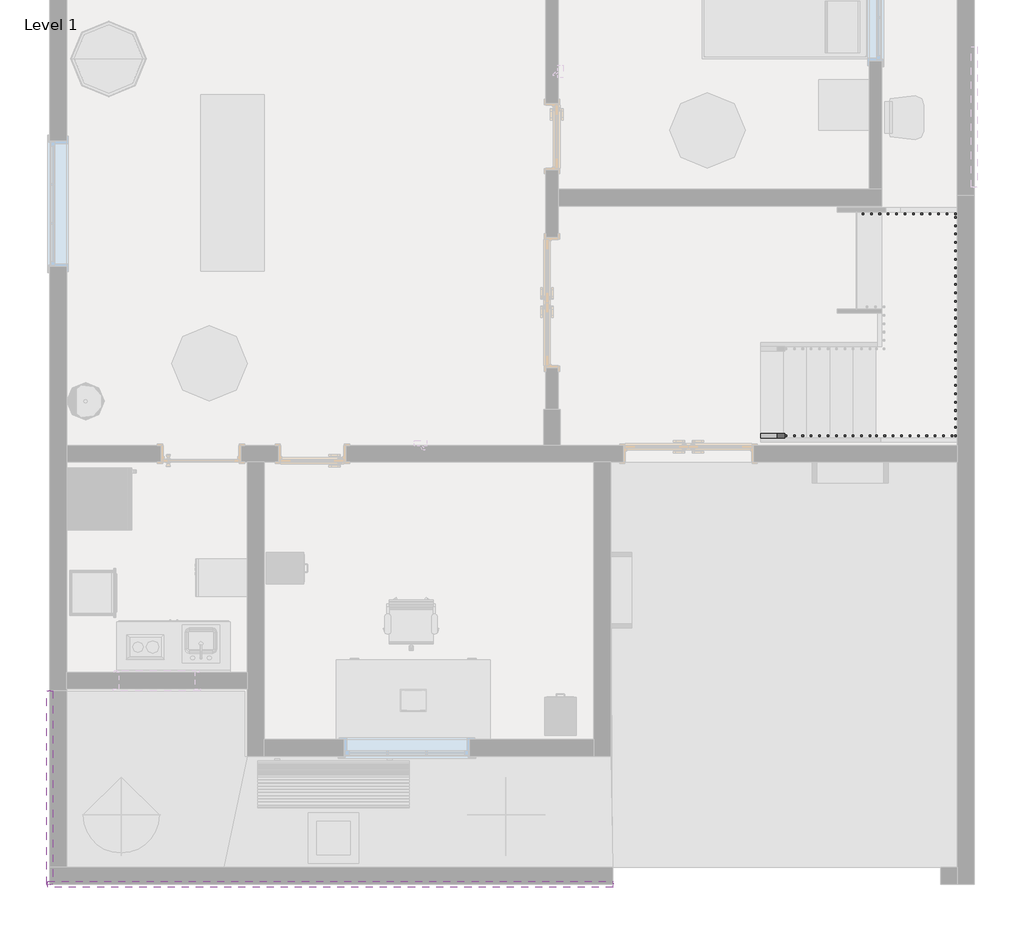
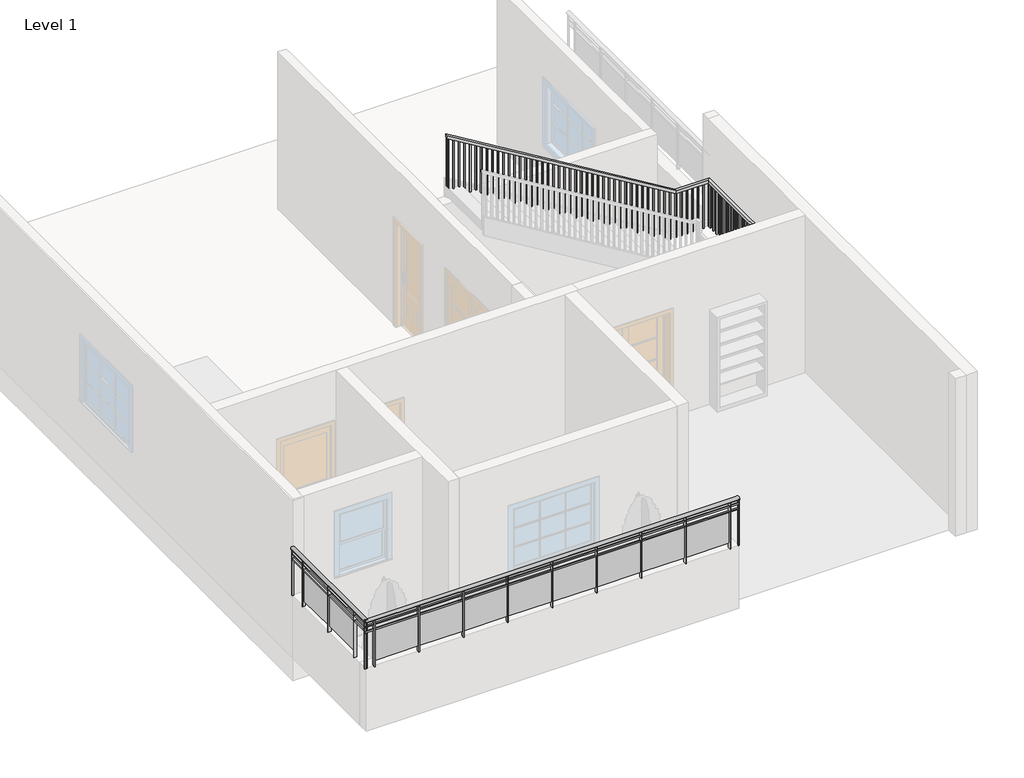
# One storey, part 2 of 4: 3 railings.
"""IFC4 building model written with IfcOpenShell, lengths in millimetres."""

from ifc_helpers import new_model, si_unit, point, frame, origin, place, context, project, spatial, polyline, ellipse_curve, trimmed, outline, extrude, faceted_brep, element, save
from ifc_brep_helpers import plane_surface, extruded_surface, advanced_brep

model = new_model("IFC4")

# Units and contexts
model_context = context("Model", 3, world=origin())
ifc_project = project(units=[si_unit("LENGTHUNIT", "METRE", prefix="MILLI")], contexts=[model_context])

# Site, building, storey
site = spatial("IfcSite", under=ifc_project)
building = spatial("IfcBuilding", under=site)
storey = spatial("IfcBuildingStorey", under=building, Name="Level 1", Elevation=0.0)

# Railings
placement = place(None, origin())
element("IfcRailing", 1, ObjectType="Glass Panel - Bottom Fill", at=placement, inside=storey, context=model_context, shape_type="SolidModel", body=[
    advanced_brep(
    [(-11727.0886283, -588.2425054, 2133.6), (-11803.2886283, -588.2425054, 2133.6), (-11727.0886283, -2925.0425054, 2133.6), (-11803.2886283, -2925.0425054, 2133.6)],
    [
        (0, 1, ellipse_curve(frame((-11765.1886283, -588.2425054, 2133.6), z_axis=(0.0, 1.0, 0.0), x_axis=(-1.0, 0.0, 0.0)), 38.1, 28.575)),
        (1, 0, ellipse_curve(frame((-11765.1886283, -588.2425054, 2133.6), z_axis=(0.0, 1.0, 0.0), x_axis=(-1.0, 0.0, 0.0)), 38.1, 28.575)),
        (2, 3, ellipse_curve(frame((-11765.1886283, -2925.0425054, 2133.6), z_axis=(0.0, -1.0, 0.0), x_axis=(-1.0, 0.0, 0.0)), 38.1, 28.575)),
        (3, 2, ellipse_curve(frame((-11765.1886283, -2925.0425054, 2133.6), z_axis=(0.0, -1.0, 0.0), x_axis=(-1.0, 0.0, 0.0)), 38.1, 28.575)),
        (0, 2),
        (3, 1),
    ],
    [
        plane_surface(frame((-11765.1886283, -588.2425054, 2133.6), z_axis=(0.0, 1.0, 0.0), x_axis=(0.0, 0.0, -1.0))),
        plane_surface(frame((-11765.1886283, -2925.0425054, 2133.6), z_axis=(0.0, -1.0, 0.0), x_axis=(0.0, 0.0, -1.0))),
        extruded_surface(trimmed(ellipse_curve(frame((-11765.1886283, -2925.0425054, 2133.6), z_axis=(0.0, 1.0, 0.0), x_axis=(-1.0, 0.0, 0.0)), 38.1, 28.575), [point((-11727.0886283, -2925.0425054, 2133.6))], [point((-11803.2886283, -2925.0425054, 2133.6))], True, "CARTESIAN"), (0.0, 2336.8, 0.0), 2336.8),
        extruded_surface(trimmed(ellipse_curve(frame((-11765.1886283, -2925.0425054, 2133.6), z_axis=(0.0, 1.0, 0.0), x_axis=(-1.0, 0.0, 0.0)), 38.1, 28.575), [point((-11803.2886283, -2925.0425054, 2133.6))], [point((-11727.0886283, -2925.0425054, 2133.6))], True, "CARTESIAN"), (0.0, 2336.8, 0.0), 2336.8),
    ],
    [
        (0, [[1, 2]]),
        (1, [[3, 4]]),
        (2, [[-1, 5, -4, 6]]),
        (3, [[-2, -6, -3, -5]]),
    ],
),
    extrude(outline(polyline([(-11777.8886283, -588.2425054), (-11752.4886283, -588.2425054), (-11752.4886283, -2925.0425054), (-11777.8886283, -2925.0425054), (-11777.8886283, -588.2425054)])), frame((0.0, 0.0, 2019.3), z_axis=(0.0, 0.0, 1.0), x_axis=(1.0, 0.0, 0.0)), (0.0, 0.0, 1.0), 25.4),
    extrude(outline(polyline([(-11777.8886283, -588.2425054), (-11752.4886283, -588.2425054), (-11752.4886283, -2925.0425054), (-11777.8886283, -2925.0425054), (-11777.8886283, -588.2425054)])), frame((0.0, 0.0, 1917.7), z_axis=(0.0, 0.0, 1.0), x_axis=(1.0, 0.0, 0.0)), (0.0, 0.0, 1.0), 25.4),
    extrude(outline(polyline([(-11790.5886283, -2563.0925054), (-11739.7886283, -2563.0925054), (-11739.7886283, -2575.7925054), (-11790.5886283, -2575.7925054), (-11790.5886283, -2563.0925054)])), frame((0.0, 0.0, 1219.2), z_axis=(0.0, 0.0, 1.0), x_axis=(1.0, 0.0, 0.0)), (0.0, 0.0, 1.0), 885.6788223),
    extrude(outline(polyline([(-11758.6534713, -1756.6425054), (-11758.6534713, -2569.4425054), (-11765.0034713, -2569.4425054), (-11765.0034713, -1756.6425054), (-11758.6534713, -1756.6425054)])), frame((0.0, 0.0, 1320.8), z_axis=(0.0, 0.0, 1.0), x_axis=(1.0, 0.0, 0.0)), (0.0, 0.0, 1.0), 596.9),
    extrude(outline(polyline([(-11790.5886283, -1750.2925054), (-11739.7886283, -1750.2925054), (-11739.7886283, -1762.9925054), (-11790.5886283, -1762.9925054), (-11790.5886283, -1750.2925054)])), frame((0.0, 0.0, 1219.2), z_axis=(0.0, 0.0, 1.0), x_axis=(1.0, 0.0, 0.0)), (0.0, 0.0, 1.0), 885.6788223),
    extrude(outline(polyline([(-11758.6534713, -943.8425054), (-11758.6534713, -1756.6425054), (-11765.0034713, -1756.6425054), (-11765.0034713, -943.8425054), (-11758.6534713, -943.8425054)])), frame((0.0, 0.0, 1320.8), z_axis=(0.0, 0.0, 1.0), x_axis=(1.0, 0.0, 0.0)), (0.0, 0.0, 1.0), 596.9),
    extrude(outline(polyline([(-11790.5886283, -937.4925054), (-11739.7886283, -937.4925054), (-11739.7886283, -950.1925054), (-11790.5886283, -950.1925054), (-11790.5886283, -937.4925054)])), frame((0.0, 0.0, 1219.2), z_axis=(0.0, 0.0, 1.0), x_axis=(1.0, 0.0, 0.0)), (0.0, 0.0, 1.0), 885.6788223),
    extrude(outline(polyline([(-11774.7136283, -2912.3425054), (-11755.6636283, -2912.3425054), (-11755.6636283, -2931.3925054), (-11774.7136283, -2931.3925054), (-11774.7136283, -2912.3425054)])), frame((0.0, 0.0, 1219.2), z_axis=(0.0, 0.0, 1.0), x_axis=(1.0, 0.0, 0.0)), (0.0, 0.0, 1.0), 885.6788223),
    extrude(outline(polyline([(-11774.7136283, -581.8925054), (-11755.6636283, -581.8925054), (-11755.6636283, -600.9425054), (-11774.7136283, -600.9425054), (-11774.7136283, -581.8925054)])), frame((0.0, 0.0, 1219.2), z_axis=(0.0, 0.0, 1.0), x_axis=(1.0, 0.0, 0.0)), (0.0, 0.0, 1.0), 885.6788223),
])
element("IfcRailing", 2, ObjectType="Glass Panel - Bottom Fill", at=placement, inside=storey, context=model_context, shape_type="SolidModel", body=[
    advanced_brep(
    [(-11790.5886283, -2886.9425054, 2133.6), (-11790.5886283, -2963.1425054, 2133.6), (-4957.9886283, -2886.9425054, 2133.6), (-4957.9886283, -2963.1425054, 2133.6)],
    [
        (0, 1, ellipse_curve(frame((-11790.5886283, -2925.0425054, 2133.6), z_axis=(-1.0, 0.0, 0.0), x_axis=(0.0, -1.0, 0.0)), 38.1, 28.575)),
        (1, 0, ellipse_curve(frame((-11790.5886283, -2925.0425054, 2133.6), z_axis=(-1.0, 0.0, 0.0), x_axis=(0.0, -1.0, 0.0)), 38.1, 28.575)),
        (2, 3, ellipse_curve(frame((-4957.9886283, -2925.0425054, 2133.6), z_axis=(1.0, 0.0, 0.0), x_axis=(0.0, -1.0, 0.0)), 38.1, 28.575)),
        (3, 2, ellipse_curve(frame((-4957.9886283, -2925.0425054, 2133.6), z_axis=(1.0, 0.0, 0.0), x_axis=(0.0, -1.0, 0.0)), 38.1, 28.575)),
        (0, 2),
        (3, 1),
    ],
    [
        plane_surface(frame((-11790.5886283, -2925.0425054, 2133.6), z_axis=(-1.0, 0.0, 0.0), x_axis=(0.0, 1.0, 0.0))),
        plane_surface(frame((-4957.9886283, -2925.0425054, 2133.6), z_axis=(1.0, 0.0, 0.0), x_axis=(0.0, 1.0, 0.0))),
        extruded_surface(trimmed(ellipse_curve(frame((-4957.9886283, -2925.0425054, 2133.6), z_axis=(-1.0, 0.0, 0.0), x_axis=(0.0, -1.0, 0.0)), 38.1, 28.575), [point((-4957.9886283, -2886.9425054, 2133.6))], [point((-4957.9886283, -2963.1425054, 2133.6))], True, "CARTESIAN"), (-6832.6, 0.0, 0.0), 6832.6),
        extruded_surface(trimmed(ellipse_curve(frame((-4957.9886283, -2925.0425054, 2133.6), z_axis=(-1.0, 0.0, 0.0), x_axis=(0.0, -1.0, 0.0)), 38.1, 28.575), [point((-4957.9886283, -2963.1425054, 2133.6))], [point((-4957.9886283, -2886.9425054, 2133.6))], True, "CARTESIAN"), (-6832.6, 0.0, 0.0), 6832.6),
    ],
    [
        (0, [[1, 2]]),
        (1, [[3, 4]]),
        (2, [[-1, 5, -4, 6]]),
        (3, [[-2, -6, -3, -5]]),
    ],
),
    extrude(outline(polyline([(-11790.5886283, -2937.7425054), (-11790.5886283, -2912.3425054), (-4957.9886283, -2912.3425054), (-4957.9886283, -2937.7425054), (-11790.5886283, -2937.7425054)])), frame((0.0, 0.0, 2019.3), z_axis=(0.0, 0.0, 1.0), x_axis=(1.0, 0.0, 0.0)), (0.0, 0.0, 1.0), 25.4),
    extrude(outline(polyline([(-11790.5886283, -2937.7425054), (-11790.5886283, -2912.3425054), (-4957.9886283, -2912.3425054), (-4957.9886283, -2937.7425054), (-11790.5886283, -2937.7425054)])), frame((0.0, 0.0, 1917.7), z_axis=(0.0, 0.0, 1.0), x_axis=(1.0, 0.0, 0.0)), (0.0, 0.0, 1.0), 25.4),
    extrude(outline(polyline([(-5129.4386283, -2950.4425054), (-5129.4386283, -2899.6425054), (-5116.7386283, -2899.6425054), (-5116.7386283, -2950.4425054), (-5129.4386283, -2950.4425054)])), frame((0.0, 0.0, 1219.2), z_axis=(0.0, 0.0, 1.0), x_axis=(1.0, 0.0, 0.0)), (0.0, 0.0, 1.0), 885.6788223),
    extrude(outline(polyline([(-5935.8886283, -2918.5073484), (-5123.0886283, -2918.5073484), (-5123.0886283, -2924.8573484), (-5935.8886283, -2924.8573484), (-5935.8886283, -2918.5073484)])), frame((0.0, 0.0, 1320.8), z_axis=(0.0, 0.0, 1.0), x_axis=(1.0, 0.0, 0.0)), (0.0, 0.0, 1.0), 596.9),
    extrude(outline(polyline([(-5942.2386283, -2950.4425054), (-5942.2386283, -2899.6425054), (-5929.5386283, -2899.6425054), (-5929.5386283, -2950.4425054), (-5942.2386283, -2950.4425054)])), frame((0.0, 0.0, 1219.2), z_axis=(0.0, 0.0, 1.0), x_axis=(1.0, 0.0, 0.0)), (0.0, 0.0, 1.0), 885.6788223),
    extrude(outline(polyline([(-6748.6886283, -2918.5073484), (-5935.8886283, -2918.5073484), (-5935.8886283, -2924.8573484), (-6748.6886283, -2924.8573484), (-6748.6886283, -2918.5073484)])), frame((0.0, 0.0, 1320.8), z_axis=(0.0, 0.0, 1.0), x_axis=(1.0, 0.0, 0.0)), (0.0, 0.0, 1.0), 596.9),
    extrude(outline(polyline([(-6755.0386283, -2950.4425054), (-6755.0386283, -2899.6425054), (-6742.3386283, -2899.6425054), (-6742.3386283, -2950.4425054), (-6755.0386283, -2950.4425054)])), frame((0.0, 0.0, 1219.2), z_axis=(0.0, 0.0, 1.0), x_axis=(1.0, 0.0, 0.0)), (0.0, 0.0, 1.0), 885.6788223),
    extrude(outline(polyline([(-7561.4886283, -2918.5073484), (-6748.6886283, -2918.5073484), (-6748.6886283, -2924.8573484), (-7561.4886283, -2924.8573484), (-7561.4886283, -2918.5073484)])), frame((0.0, 0.0, 1320.8), z_axis=(0.0, 0.0, 1.0), x_axis=(1.0, 0.0, 0.0)), (0.0, 0.0, 1.0), 596.9),
    extrude(outline(polyline([(-7567.8386283, -2950.4425054), (-7567.8386283, -2899.6425054), (-7555.1386283, -2899.6425054), (-7555.1386283, -2950.4425054), (-7567.8386283, -2950.4425054)])), frame((0.0, 0.0, 1219.2), z_axis=(0.0, 0.0, 1.0), x_axis=(1.0, 0.0, 0.0)), (0.0, 0.0, 1.0), 885.6788223),
    extrude(outline(polyline([(-8374.2886283, -2918.5073484), (-7561.4886283, -2918.5073484), (-7561.4886283, -2924.8573484), (-8374.2886283, -2924.8573484), (-8374.2886283, -2918.5073484)])), frame((0.0, 0.0, 1320.8), z_axis=(0.0, 0.0, 1.0), x_axis=(1.0, 0.0, 0.0)), (0.0, 0.0, 1.0), 596.9),
    extrude(outline(polyline([(-8380.6386283, -2950.4425054), (-8380.6386283, -2899.6425054), (-8367.9386283, -2899.6425054), (-8367.9386283, -2950.4425054), (-8380.6386283, -2950.4425054)])), frame((0.0, 0.0, 1219.2), z_axis=(0.0, 0.0, 1.0), x_axis=(1.0, 0.0, 0.0)), (0.0, 0.0, 1.0), 885.6788223),
    extrude(outline(polyline([(-9187.0886283, -2918.5073484), (-8374.2886283, -2918.5073484), (-8374.2886283, -2924.8573484), (-9187.0886283, -2924.8573484), (-9187.0886283, -2918.5073484)])), frame((0.0, 0.0, 1320.8), z_axis=(0.0, 0.0, 1.0), x_axis=(1.0, 0.0, 0.0)), (0.0, 0.0, 1.0), 596.9),
    extrude(outline(polyline([(-9193.4386283, -2950.4425054), (-9193.4386283, -2899.6425054), (-9180.7386283, -2899.6425054), (-9180.7386283, -2950.4425054), (-9193.4386283, -2950.4425054)])), frame((0.0, 0.0, 1219.2), z_axis=(0.0, 0.0, 1.0), x_axis=(1.0, 0.0, 0.0)), (0.0, 0.0, 1.0), 885.6788223),
    extrude(outline(polyline([(-9999.8886283, -2918.5073484), (-9187.0886283, -2918.5073484), (-9187.0886283, -2924.8573484), (-9999.8886283, -2924.8573484), (-9999.8886283, -2918.5073484)])), frame((0.0, 0.0, 1320.8), z_axis=(0.0, 0.0, 1.0), x_axis=(1.0, 0.0, 0.0)), (0.0, 0.0, 1.0), 596.9),
    extrude(outline(polyline([(-10006.2386283, -2950.4425054), (-10006.2386283, -2899.6425054), (-9993.5386283, -2899.6425054), (-9993.5386283, -2950.4425054), (-10006.2386283, -2950.4425054)])), frame((0.0, 0.0, 1219.2), z_axis=(0.0, 0.0, 1.0), x_axis=(1.0, 0.0, 0.0)), (0.0, 0.0, 1.0), 885.6788223),
    extrude(outline(polyline([(-10812.6886283, -2918.5073484), (-9999.8886283, -2918.5073484), (-9999.8886283, -2924.8573484), (-10812.6886283, -2924.8573484), (-10812.6886283, -2918.5073484)])), frame((0.0, 0.0, 1320.8), z_axis=(0.0, 0.0, 1.0), x_axis=(1.0, 0.0, 0.0)), (0.0, 0.0, 1.0), 596.9),
    extrude(outline(polyline([(-10819.0386283, -2950.4425054), (-10819.0386283, -2899.6425054), (-10806.3386283, -2899.6425054), (-10806.3386283, -2950.4425054), (-10819.0386283, -2950.4425054)])), frame((0.0, 0.0, 1219.2), z_axis=(0.0, 0.0, 1.0), x_axis=(1.0, 0.0, 0.0)), (0.0, 0.0, 1.0), 885.6788223),
    extrude(outline(polyline([(-11625.4886283, -2918.5073484), (-10812.6886283, -2918.5073484), (-10812.6886283, -2924.8573484), (-11625.4886283, -2924.8573484), (-11625.4886283, -2918.5073484)])), frame((0.0, 0.0, 1320.8), z_axis=(0.0, 0.0, 1.0), x_axis=(1.0, 0.0, 0.0)), (0.0, 0.0, 1.0), 596.9),
    extrude(outline(polyline([(-11631.8386283, -2950.4425054), (-11631.8386283, -2899.6425054), (-11619.1386283, -2899.6425054), (-11619.1386283, -2950.4425054), (-11631.8386283, -2950.4425054)])), frame((0.0, 0.0, 1219.2), z_axis=(0.0, 0.0, 1.0), x_axis=(1.0, 0.0, 0.0)), (0.0, 0.0, 1.0), 885.6788223),
    extrude(outline(polyline([(-4970.6886283, -2934.5675054), (-4970.6886283, -2915.5175054), (-4951.6386283, -2915.5175054), (-4951.6386283, -2934.5675054), (-4970.6886283, -2934.5675054)])), frame((0.0, 0.0, 1219.2), z_axis=(0.0, 0.0, 1.0), x_axis=(1.0, 0.0, 0.0)), (0.0, 0.0, 1.0), 885.6788223),
    extrude(outline(polyline([(-11796.9386283, -2934.5675054), (-11796.9386283, -2915.5175054), (-11777.8886283, -2915.5175054), (-11777.8886283, -2934.5675054), (-11796.9386283, -2934.5675054)])), frame((0.0, 0.0, 1219.2), z_axis=(0.0, 0.0, 1.0), x_axis=(1.0, 0.0, 0.0)), (0.0, 0.0, 1.0), 885.6788223),
])
element("IfcRailing", 3, ObjectType="Handrail - Rectangular", at=placement, inside=storey, context=model_context, shape_type="SolidModel", body=[
    faceted_brep([(-3170.5888787, 2525.6939653, 1083.7333333), (-3170.5888787, 2525.6939653, 1024.3318731), (-3170.5888787, 2474.8939653, 1024.3318731), (-3170.5888787, 2474.8939653, 1083.7333333), (-1773.5888787, 2525.6939653, 1930.4), (-1759.3964693, 2525.6939653, 1879.6), (-1759.3964693, 2474.8939653, 1879.6), (-1773.5888787, 2474.8939653, 1930.4), (-843.1886283, 2525.6939653, 1930.4), (-843.1886283, 2525.6939653, 1879.6), (-792.3886283, 2474.8939653, 1879.6), (-792.3886283, 2474.8939653, 1930.4), (-843.1886283, 5156.0078573, 1930.4), (-843.1886283, 5156.0078573, 1879.6), (-792.3886283, 5206.8078573, 1879.6), (-792.3886283, 5206.8078573, 1930.4), (-1427.3886283, 5156.0078573, 1930.4), (-1441.5810377, 5156.0078573, 1879.6), (-1441.5810377, 5206.8078573, 1879.6), (-1427.3886283, 5206.8078573, 1930.4), (-5618.3886283, 5156.0078573, 4470.4), (-5618.3886283, 5206.8078573, 4470.4), (-5618.3886283, 5206.8078573, 4410.9985397), (-5618.3886283, 5156.0078573, 4410.9985397)], [[[0, 1, 2, 3]], [[1, 0, 4, 5]], [[2, 1, 5, 6]], [[3, 2, 6, 7]], [[0, 3, 7, 4]], [[5, 4, 8, 9]], [[6, 5, 9, 10]], [[7, 6, 10, 11]], [[4, 7, 11, 8]], [[9, 8, 12, 13]], [[10, 9, 13, 14]], [[11, 10, 14, 15]], [[8, 11, 15, 12]], [[13, 12, 16, 17]], [[14, 13, 17, 18]], [[15, 14, 18, 19]], [[12, 15, 19, 16]], [[20, 21, 22, 23]], [[17, 16, 20, 23]], [[18, 17, 23, 22]], [[19, 18, 22, 21]], [[16, 19, 21, 20]]]),
    extrude(outline(polyline([(4389.8318731, -5583.4636283), (4401.3773276, -5602.5136283), (3386.6666667, -5602.5136283), (3386.6666667, -5583.4636283), (4389.8318731, -5583.4636283)])), frame((0.0, 5171.8828573, 0.0), z_axis=(0.0, 1.0, 0.0), x_axis=(0.0, 0.0, 1.0)), (0.0, 0.0, 1.0), 19.05),
    extrude(outline(polyline([(4328.2561155, -5481.8636283), (4339.80157, -5500.9136283), (3386.6666667, -5500.9136283), (3386.6666667, -5481.8636283), (4328.2561155, -5481.8636283)])), frame((0.0, 5171.8828573, 0.0), z_axis=(0.0, 1.0, 0.0), x_axis=(0.0, 0.0, 1.0)), (0.0, 0.0, 1.0), 19.05),
    extrude(outline(polyline([(4266.6803579, -5380.2636283), (4278.2258125, -5399.3136283), (3386.6666667, -5399.3136283), (3386.6666667, -5380.2636283), (4266.6803579, -5380.2636283)])), frame((0.0, 5171.8828573, 0.0), z_axis=(0.0, 1.0, 0.0), x_axis=(0.0, 0.0, 1.0)), (0.0, 0.0, 1.0), 19.05),
    extrude(outline(polyline([(4205.1046004, -5278.6636283), (4216.6500549, -5297.7136283), (3217.3333333, -5297.7136283), (3217.3333333, -5278.6636283), (4205.1046004, -5278.6636283)])), frame((0.0, 5171.8828573, 0.0), z_axis=(0.0, 1.0, 0.0), x_axis=(0.0, 0.0, 1.0)), (0.0, 0.0, 1.0), 19.05),
    extrude(outline(polyline([(4143.5288428, -5177.0636283), (4155.0742973, -5196.1136283), (3217.3333333, -5196.1136283), (3217.3333333, -5177.0636283), (4143.5288428, -5177.0636283)])), frame((0.0, 5171.8828573, 0.0), z_axis=(0.0, 1.0, 0.0), x_axis=(0.0, 0.0, 1.0)), (0.0, 0.0, 1.0), 19.05),
    extrude(outline(polyline([(4081.9530852, -5075.4636283), (4093.4985397, -5094.5136283), (3217.3333333, -5094.5136283), (3217.3333333, -5075.4636283), (4081.9530852, -5075.4636283)])), frame((0.0, 5171.8828573, 0.0), z_axis=(0.0, 1.0, 0.0), x_axis=(0.0, 0.0, 1.0)), (0.0, 0.0, 1.0), 19.05),
    extrude(outline(polyline([(4020.3773276, -4973.8636283), (4031.9227822, -4992.9136283), (3048.0, -4992.9136283), (3048.0, -4973.8636283), (4020.3773276, -4973.8636283)])), frame((0.0, 5171.8828573, 0.0), z_axis=(0.0, 1.0, 0.0), x_axis=(0.0, 0.0, 1.0)), (0.0, 0.0, 1.0), 19.05),
    extrude(outline(polyline([(3958.80157, -4872.2636283), (3970.3470246, -4891.3136283), (3048.0, -4891.3136283), (3048.0, -4872.2636283), (3958.80157, -4872.2636283)])), frame((0.0, 5171.8828573, 0.0), z_axis=(0.0, 1.0, 0.0), x_axis=(0.0, 0.0, 1.0)), (0.0, 0.0, 1.0), 19.05),
    extrude(outline(polyline([(3897.2258125, -4770.6636283), (3908.771267, -4789.7136283), (3048.0, -4789.7136283), (3048.0, -4770.6636283), (3897.2258125, -4770.6636283)])), frame((0.0, 5171.8828573, 0.0), z_axis=(0.0, 1.0, 0.0), x_axis=(0.0, 0.0, 1.0)), (0.0, 0.0, 1.0), 19.05),
    extrude(outline(polyline([(3835.6500549, -4669.0636283), (3847.1955094, -4688.1136283), (2878.6666667, -4688.1136283), (2878.6666667, -4669.0636283), (3835.6500549, -4669.0636283)])), frame((0.0, 5171.8828573, 0.0), z_axis=(0.0, 1.0, 0.0), x_axis=(0.0, 0.0, 1.0)), (0.0, 0.0, 1.0), 19.05),
    extrude(outline(polyline([(3774.0742973, -4567.4636283), (3785.6197519, -4586.5136283), (2878.6666667, -4586.5136283), (2878.6666667, -4567.4636283), (3774.0742973, -4567.4636283)])), frame((0.0, 5171.8828573, 0.0), z_axis=(0.0, 1.0, 0.0), x_axis=(0.0, 0.0, 1.0)), (0.0, 0.0, 1.0), 19.05),
    extrude(outline(polyline([(3712.4985397, -4465.8636283), (3724.0439943, -4484.9136283), (2709.3333333, -4484.9136283), (2709.3333333, -4465.8636283), (3712.4985397, -4465.8636283)])), frame((0.0, 5171.8828573, 0.0), z_axis=(0.0, 1.0, 0.0), x_axis=(0.0, 0.0, 1.0)), (0.0, 0.0, 1.0), 19.05),
    extrude(outline(polyline([(3650.9227822, -4364.2636283), (3662.4682367, -4383.3136283), (2709.3333333, -4383.3136283), (2709.3333333, -4364.2636283), (3650.9227822, -4364.2636283)])), frame((0.0, 5171.8828573, 0.0), z_axis=(0.0, 1.0, 0.0), x_axis=(0.0, 0.0, 1.0)), (0.0, 0.0, 1.0), 19.05),
    extrude(outline(polyline([(3589.3470246, -4262.6636283), (3600.8924791, -4281.7136283), (2709.3333333, -4281.7136283), (2709.3333333, -4262.6636283), (3589.3470246, -4262.6636283)])), frame((0.0, 5171.8828573, 0.0), z_axis=(0.0, 1.0, 0.0), x_axis=(0.0, 0.0, 1.0)), (0.0, 0.0, 1.0), 19.05),
    extrude(outline(polyline([(3527.771267, -4161.0636283), (3539.3167216, -4180.1136283), (2540.0, -4180.1136283), (2540.0, -4161.0636283), (3527.771267, -4161.0636283)])), frame((0.0, 5171.8828573, 0.0), z_axis=(0.0, 1.0, 0.0), x_axis=(0.0, 0.0, 1.0)), (0.0, 0.0, 1.0), 19.05),
    extrude(outline(polyline([(3466.1955094, -4059.4636283), (3477.740964, -4078.5136283), (2540.0, -4078.5136283), (2540.0, -4059.4636283), (3466.1955094, -4059.4636283)])), frame((0.0, 5171.8828573, 0.0), z_axis=(0.0, 1.0, 0.0), x_axis=(0.0, 0.0, 1.0)), (0.0, 0.0, 1.0), 19.05),
    extrude(outline(polyline([(3404.6197519, -3957.8636283), (3416.1652064, -3976.9136283), (2540.0, -3976.9136283), (2540.0, -3957.8636283), (3404.6197519, -3957.8636283)])), frame((0.0, 5171.8828573, 0.0), z_axis=(0.0, 1.0, 0.0), x_axis=(0.0, 0.0, 1.0)), (0.0, 0.0, 1.0), 19.05),
    extrude(outline(polyline([(3343.0439943, -3856.2636283), (3354.5894488, -3875.3136283), (2370.6666667, -3875.3136283), (2370.6666667, -3856.2636283), (3343.0439943, -3856.2636283)])), frame((0.0, 5171.8828573, 0.0), z_axis=(0.0, 1.0, 0.0), x_axis=(0.0, 0.0, 1.0)), (0.0, 0.0, 1.0), 19.05),
    extrude(outline(polyline([(3281.4682367, -3754.6636283), (3293.0136913, -3773.7136283), (2370.6666667, -3773.7136283), (2370.6666667, -3754.6636283), (3281.4682367, -3754.6636283)])), frame((0.0, 5171.8828573, 0.0), z_axis=(0.0, 1.0, 0.0), x_axis=(0.0, 0.0, 1.0)), (0.0, 0.0, 1.0), 19.05),
    extrude(outline(polyline([(3219.8924791, -3653.0636283), (3231.4379337, -3672.1136283), (2370.6666667, -3672.1136283), (2370.6666667, -3653.0636283), (3219.8924791, -3653.0636283)])), frame((0.0, 5171.8828573, 0.0), z_axis=(0.0, 1.0, 0.0), x_axis=(0.0, 0.0, 1.0)), (0.0, 0.0, 1.0), 19.05),
    extrude(outline(polyline([(3158.3167216, -3551.4636283), (3169.8621761, -3570.5136283), (2201.3333333, -3570.5136283), (2201.3333333, -3551.4636283), (3158.3167216, -3551.4636283)])), frame((0.0, 5171.8828573, 0.0), z_axis=(0.0, 1.0, 0.0), x_axis=(0.0, 0.0, 1.0)), (0.0, 0.0, 1.0), 19.05),
    extrude(outline(polyline([(3096.740964, -3449.8636283), (3108.2864185, -3468.9136283), (2201.3333333, -3468.9136283), (2201.3333333, -3449.8636283), (3096.740964, -3449.8636283)])), frame((0.0, 5171.8828573, 0.0), z_axis=(0.0, 1.0, 0.0), x_axis=(0.0, 0.0, 1.0)), (0.0, 0.0, 1.0), 19.05),
    extrude(outline(polyline([(3035.1652064, -3348.2636283), (3046.710661, -3367.3136283), (2032.0, -3367.3136283), (2032.0, -3348.2636283), (3035.1652064, -3348.2636283)])), frame((0.0, 5171.8828573, 0.0), z_axis=(0.0, 1.0, 0.0), x_axis=(0.0, 0.0, 1.0)), (0.0, 0.0, 1.0), 19.05),
    extrude(outline(polyline([(2973.5894488, -3246.6636283), (2985.1349034, -3265.7136283), (2032.0, -3265.7136283), (2032.0, -3246.6636283), (2973.5894488, -3246.6636283)])), frame((0.0, 5171.8828573, 0.0), z_axis=(0.0, 1.0, 0.0), x_axis=(0.0, 0.0, 1.0)), (0.0, 0.0, 1.0), 19.05),
    extrude(outline(polyline([(2912.0136913, -3145.0636283), (2923.5591458, -3164.1136283), (2032.0, -3164.1136283), (2032.0, -3145.0636283), (2912.0136913, -3145.0636283)])), frame((0.0, 5171.8828573, 0.0), z_axis=(0.0, 1.0, 0.0), x_axis=(0.0, 0.0, 1.0)), (0.0, 0.0, 1.0), 19.05),
    extrude(outline(polyline([(2850.4379337, -3043.4636283), (2861.9833882, -3062.5136283), (1862.6666667, -3062.5136283), (1862.6666667, -3043.4636283), (2850.4379337, -3043.4636283)])), frame((0.0, 5171.8828573, 0.0), z_axis=(0.0, 1.0, 0.0), x_axis=(0.0, 0.0, 1.0)), (0.0, 0.0, 1.0), 19.05),
    extrude(outline(polyline([(2788.8621761, -2941.8636283), (2800.4076307, -2960.9136283), (1862.6666667, -2960.9136283), (1862.6666667, -2941.8636283), (2788.8621761, -2941.8636283)])), frame((0.0, 5171.8828573, 0.0), z_axis=(0.0, 1.0, 0.0), x_axis=(0.0, 0.0, 1.0)), (0.0, 0.0, 1.0), 19.05),
    extrude(outline(polyline([(2727.2864185, -2840.2636283), (2738.8318731, -2859.3136283), (1862.6666667, -2859.3136283), (1862.6666667, -2840.2636283), (2727.2864185, -2840.2636283)])), frame((0.0, 5171.8828573, 0.0), z_axis=(0.0, 1.0, 0.0), x_axis=(0.0, 0.0, 1.0)), (0.0, 0.0, 1.0), 19.05),
    extrude(outline(polyline([(2665.710661, -2738.6636283), (2677.2561155, -2757.7136283), (1693.3333333, -2757.7136283), (1693.3333333, -2738.6636283), (2665.710661, -2738.6636283)])), frame((0.0, 5171.8828573, 0.0), z_axis=(0.0, 1.0, 0.0), x_axis=(0.0, 0.0, 1.0)), (0.0, 0.0, 1.0), 19.05),
    extrude(outline(polyline([(2604.1349034, -2637.0636283), (2615.6803579, -2656.1136283), (1693.3333333, -2656.1136283), (1693.3333333, -2637.0636283), (2604.1349034, -2637.0636283)])), frame((0.0, 5171.8828573, 0.0), z_axis=(0.0, 1.0, 0.0), x_axis=(0.0, 0.0, 1.0)), (0.0, 0.0, 1.0), 19.05),
    extrude(outline(polyline([(2542.5591458, -2535.4636283), (2554.1046004, -2554.5136283), (1693.3333333, -2554.5136283), (1693.3333333, -2535.4636283), (2542.5591458, -2535.4636283)])), frame((0.0, 5171.8828573, 0.0), z_axis=(0.0, 1.0, 0.0), x_axis=(0.0, 0.0, 1.0)), (0.0, 0.0, 1.0), 19.05),
    extrude(outline(polyline([(2480.9833882, -2433.8636283), (2492.5288428, -2452.9136283), (1524.0, -2452.9136283), (1524.0, -2433.8636283), (2480.9833882, -2433.8636283)])), frame((0.0, 5171.8828573, 0.0), z_axis=(0.0, 1.0, 0.0), x_axis=(0.0, 0.0, 1.0)), (0.0, 0.0, 1.0), 19.05),
    extrude(outline(polyline([(2419.4076307, -2332.2636283), (2430.9530852, -2351.3136283), (1524.0, -2351.3136283), (1524.0, -2332.2636283), (2419.4076307, -2332.2636283)])), frame((0.0, 5171.8828573, 0.0), z_axis=(0.0, 1.0, 0.0), x_axis=(0.0, 0.0, 1.0)), (0.0, 0.0, 1.0), 19.05),
    extrude(outline(polyline([(2357.8318731, -2230.6636283), (2369.3773276, -2249.7136283), (1354.6666667, -2249.7136283), (1354.6666667, -2230.6636283), (2357.8318731, -2230.6636283)])), frame((0.0, 5171.8828573, 0.0), z_axis=(0.0, 1.0, 0.0), x_axis=(0.0, 0.0, 1.0)), (0.0, 0.0, 1.0), 19.05),
    extrude(outline(polyline([(2296.2561155, -2129.0636283), (2307.80157, -2148.1136283), (1354.6666667, -2148.1136283), (1354.6666667, -2129.0636283), (2296.2561155, -2129.0636283)])), frame((0.0, 5171.8828573, 0.0), z_axis=(0.0, 1.0, 0.0), x_axis=(0.0, 0.0, 1.0)), (0.0, 0.0, 1.0), 19.05),
    extrude(outline(polyline([(2234.6803579, -2027.4636283), (2246.2258125, -2046.5136283), (1354.6666667, -2046.5136283), (1354.6666667, -2027.4636283), (2234.6803579, -2027.4636283)])), frame((0.0, 5171.8828573, 0.0), z_axis=(0.0, 1.0, 0.0), x_axis=(0.0, 0.0, 1.0)), (0.0, 0.0, 1.0), 19.05),
    extrude(outline(polyline([(2173.1046004, -1925.8636283), (2184.6500549, -1944.9136283), (1185.3333333, -1944.9136283), (1185.3333333, -1925.8636283), (2173.1046004, -1925.8636283)])), frame((0.0, 5171.8828573, 0.0), z_axis=(0.0, 1.0, 0.0), x_axis=(0.0, 0.0, 1.0)), (0.0, 0.0, 1.0), 19.05),
    extrude(outline(polyline([(2111.5288428, -1824.2636283), (2123.0742973, -1843.3136283), (1185.3333333, -1843.3136283), (1185.3333333, -1824.2636283), (2111.5288428, -1824.2636283)])), frame((0.0, 5171.8828573, 0.0), z_axis=(0.0, 1.0, 0.0), x_axis=(0.0, 0.0, 1.0)), (0.0, 0.0, 1.0), 19.05),
    extrude(outline(polyline([(2049.9530852, -1722.6636283), (2061.4985397, -1741.7136283), (1185.3333333, -1741.7136283), (1185.3333333, -1722.6636283), (2049.9530852, -1722.6636283)])), frame((0.0, 5171.8828573, 0.0), z_axis=(0.0, 1.0, 0.0), x_axis=(0.0, 0.0, 1.0)), (0.0, 0.0, 1.0), 19.05),
    extrude(outline(polyline([(1988.3773276, -1621.0636283), (1999.9227822, -1640.1136283), (1016.0, -1640.1136283), (1016.0, -1621.0636283), (1988.3773276, -1621.0636283)])), frame((0.0, 5171.8828573, 0.0), z_axis=(0.0, 1.0, 0.0), x_axis=(0.0, 0.0, 1.0)), (0.0, 0.0, 1.0), 19.05),
    extrude(outline(polyline([(1926.80157, -1519.4636283), (1938.3470246, -1538.5136283), (1016.0, -1538.5136283), (1016.0, -1519.4636283), (1926.80157, -1519.4636283)])), frame((0.0, 5171.8828573, 0.0), z_axis=(0.0, 1.0, 0.0), x_axis=(0.0, 0.0, 1.0)), (0.0, 0.0, 1.0), 19.05),
    extrude(outline(polyline([(-1316.2636283, 5190.9328573), (-1316.2636283, 5171.8828573), (-1335.3136283, 5171.8828573), (-1335.3136283, 5190.9328573), (-1316.2636283, 5190.9328573)])), frame((0.0, 0.0, 1016.0), z_axis=(0.0, 0.0, 1.0), x_axis=(1.0, 0.0, 0.0)), (0.0, 0.0, 1.0), 863.6),
    extrude(outline(polyline([(-1214.6636283, 5190.9328573), (-1214.6636283, 5171.8828573), (-1233.7136283, 5171.8828573), (-1233.7136283, 5190.9328573), (-1214.6636283, 5190.9328573)])), frame((0.0, 0.0, 1016.0), z_axis=(0.0, 0.0, 1.0), x_axis=(1.0, 0.0, 0.0)), (0.0, 0.0, 1.0), 863.6),
    extrude(outline(polyline([(-1113.0636283, 5190.9328573), (-1113.0636283, 5171.8828573), (-1132.1136283, 5171.8828573), (-1132.1136283, 5190.9328573), (-1113.0636283, 5190.9328573)])), frame((0.0, 0.0, 1016.0), z_axis=(0.0, 0.0, 1.0), x_axis=(1.0, 0.0, 0.0)), (0.0, 0.0, 1.0), 863.6),
    extrude(outline(polyline([(-1011.4636283, 5190.9328573), (-1011.4636283, 5171.8828573), (-1030.5136283, 5171.8828573), (-1030.5136283, 5190.9328573), (-1011.4636283, 5190.9328573)])), frame((0.0, 0.0, 1016.0), z_axis=(0.0, 0.0, 1.0), x_axis=(1.0, 0.0, 0.0)), (0.0, 0.0, 1.0), 863.6),
    extrude(outline(polyline([(-909.8636283, 5190.9328573), (-909.8636283, 5171.8828573), (-928.9136283, 5171.8828573), (-928.9136283, 5190.9328573), (-909.8636283, 5190.9328573)])), frame((0.0, 0.0, 1016.0), z_axis=(0.0, 0.0, 1.0), x_axis=(1.0, 0.0, 0.0)), (0.0, 0.0, 1.0), 863.6),
    extrude(outline(polyline([(-808.2636283, 5132.3689653), (-827.3136283, 5132.3689653), (-827.3136283, 5151.4189653), (-808.2636283, 5151.4189653), (-808.2636283, 5132.3689653)])), frame((0.0, 0.0, 1016.0), z_axis=(0.0, 0.0, 1.0), x_axis=(1.0, 0.0, 0.0)), (0.0, 0.0, 1.0), 863.6),
    extrude(outline(polyline([(-808.2636283, 5030.7689653), (-827.3136283, 5030.7689653), (-827.3136283, 5049.8189653), (-808.2636283, 5049.8189653), (-808.2636283, 5030.7689653)])), frame((0.0, 0.0, 1016.0), z_axis=(0.0, 0.0, 1.0), x_axis=(1.0, 0.0, 0.0)), (0.0, 0.0, 1.0), 863.6),
    extrude(outline(polyline([(-808.2636283, 4929.1689653), (-827.3136283, 4929.1689653), (-827.3136283, 4948.2189653), (-808.2636283, 4948.2189653), (-808.2636283, 4929.1689653)])), frame((0.0, 0.0, 1016.0), z_axis=(0.0, 0.0, 1.0), x_axis=(1.0, 0.0, 0.0)), (0.0, 0.0, 1.0), 863.6),
    extrude(outline(polyline([(-808.2636283, 4827.5689653), (-827.3136283, 4827.5689653), (-827.3136283, 4846.6189653), (-808.2636283, 4846.6189653), (-808.2636283, 4827.5689653)])), frame((0.0, 0.0, 1016.0), z_axis=(0.0, 0.0, 1.0), x_axis=(1.0, 0.0, 0.0)), (0.0, 0.0, 1.0), 863.6),
    extrude(outline(polyline([(-808.2636283, 4725.9689653), (-827.3136283, 4725.9689653), (-827.3136283, 4745.0189653), (-808.2636283, 4745.0189653), (-808.2636283, 4725.9689653)])), frame((0.0, 0.0, 1016.0), z_axis=(0.0, 0.0, 1.0), x_axis=(1.0, 0.0, 0.0)), (0.0, 0.0, 1.0), 863.6),
    extrude(outline(polyline([(-808.2636283, 4624.3689653), (-827.3136283, 4624.3689653), (-827.3136283, 4643.4189653), (-808.2636283, 4643.4189653), (-808.2636283, 4624.3689653)])), frame((0.0, 0.0, 1016.0), z_axis=(0.0, 0.0, 1.0), x_axis=(1.0, 0.0, 0.0)), (0.0, 0.0, 1.0), 863.6),
    extrude(outline(polyline([(-808.2636283, 4522.7689653), (-827.3136283, 4522.7689653), (-827.3136283, 4541.8189653), (-808.2636283, 4541.8189653), (-808.2636283, 4522.7689653)])), frame((0.0, 0.0, 1016.0), z_axis=(0.0, 0.0, 1.0), x_axis=(1.0, 0.0, 0.0)), (0.0, 0.0, 1.0), 863.6),
    extrude(outline(polyline([(-808.2636283, 4421.1689653), (-827.3136283, 4421.1689653), (-827.3136283, 4440.2189653), (-808.2636283, 4440.2189653), (-808.2636283, 4421.1689653)])), frame((0.0, 0.0, 1016.0), z_axis=(0.0, 0.0, 1.0), x_axis=(1.0, 0.0, 0.0)), (0.0, 0.0, 1.0), 863.6),
    extrude(outline(polyline([(-808.2636283, 4319.5689653), (-827.3136283, 4319.5689653), (-827.3136283, 4338.6189653), (-808.2636283, 4338.6189653), (-808.2636283, 4319.5689653)])), frame((0.0, 0.0, 1016.0), z_axis=(0.0, 0.0, 1.0), x_axis=(1.0, 0.0, 0.0)), (0.0, 0.0, 1.0), 863.6),
    extrude(outline(polyline([(-808.2636283, 4217.9689653), (-827.3136283, 4217.9689653), (-827.3136283, 4237.0189653), (-808.2636283, 4237.0189653), (-808.2636283, 4217.9689653)])), frame((0.0, 0.0, 1016.0), z_axis=(0.0, 0.0, 1.0), x_axis=(1.0, 0.0, 0.0)), (0.0, 0.0, 1.0), 863.6),
    extrude(outline(polyline([(-808.2636283, 4116.3689653), (-827.3136283, 4116.3689653), (-827.3136283, 4135.4189653), (-808.2636283, 4135.4189653), (-808.2636283, 4116.3689653)])), frame((0.0, 0.0, 1016.0), z_axis=(0.0, 0.0, 1.0), x_axis=(1.0, 0.0, 0.0)), (0.0, 0.0, 1.0), 863.6),
    extrude(outline(polyline([(-808.2636283, 4014.7689653), (-827.3136283, 4014.7689653), (-827.3136283, 4033.8189653), (-808.2636283, 4033.8189653), (-808.2636283, 4014.7689653)])), frame((0.0, 0.0, 1016.0), z_axis=(0.0, 0.0, 1.0), x_axis=(1.0, 0.0, 0.0)), (0.0, 0.0, 1.0), 863.6),
    extrude(outline(polyline([(-808.2636283, 3913.1689653), (-827.3136283, 3913.1689653), (-827.3136283, 3932.2189653), (-808.2636283, 3932.2189653), (-808.2636283, 3913.1689653)])), frame((0.0, 0.0, 1016.0), z_axis=(0.0, 0.0, 1.0), x_axis=(1.0, 0.0, 0.0)), (0.0, 0.0, 1.0), 863.6),
    extrude(outline(polyline([(-808.2636283, 3811.5689653), (-827.3136283, 3811.5689653), (-827.3136283, 3830.6189653), (-808.2636283, 3830.6189653), (-808.2636283, 3811.5689653)])), frame((0.0, 0.0, 1016.0), z_axis=(0.0, 0.0, 1.0), x_axis=(1.0, 0.0, 0.0)), (0.0, 0.0, 1.0), 863.6),
    extrude(outline(polyline([(-808.2636283, 3709.9689653), (-827.3136283, 3709.9689653), (-827.3136283, 3729.0189653), (-808.2636283, 3729.0189653), (-808.2636283, 3709.9689653)])), frame((0.0, 0.0, 1016.0), z_axis=(0.0, 0.0, 1.0), x_axis=(1.0, 0.0, 0.0)), (0.0, 0.0, 1.0), 863.6),
    extrude(outline(polyline([(-808.2636283, 3608.3689653), (-827.3136283, 3608.3689653), (-827.3136283, 3627.4189653), (-808.2636283, 3627.4189653), (-808.2636283, 3608.3689653)])), frame((0.0, 0.0, 1016.0), z_axis=(0.0, 0.0, 1.0), x_axis=(1.0, 0.0, 0.0)), (0.0, 0.0, 1.0), 863.6),
    extrude(outline(polyline([(-808.2636283, 3506.7689653), (-827.3136283, 3506.7689653), (-827.3136283, 3525.8189653), (-808.2636283, 3525.8189653), (-808.2636283, 3506.7689653)])), frame((0.0, 0.0, 1016.0), z_axis=(0.0, 0.0, 1.0), x_axis=(1.0, 0.0, 0.0)), (0.0, 0.0, 1.0), 863.6),
    extrude(outline(polyline([(-808.2636283, 3405.1689653), (-827.3136283, 3405.1689653), (-827.3136283, 3424.2189653), (-808.2636283, 3424.2189653), (-808.2636283, 3405.1689653)])), frame((0.0, 0.0, 1016.0), z_axis=(0.0, 0.0, 1.0), x_axis=(1.0, 0.0, 0.0)), (0.0, 0.0, 1.0), 863.6),
    extrude(outline(polyline([(-808.2636283, 3303.5689653), (-827.3136283, 3303.5689653), (-827.3136283, 3322.6189653), (-808.2636283, 3322.6189653), (-808.2636283, 3303.5689653)])), frame((0.0, 0.0, 1016.0), z_axis=(0.0, 0.0, 1.0), x_axis=(1.0, 0.0, 0.0)), (0.0, 0.0, 1.0), 863.6),
    extrude(outline(polyline([(-808.2636283, 3201.9689653), (-827.3136283, 3201.9689653), (-827.3136283, 3221.0189653), (-808.2636283, 3221.0189653), (-808.2636283, 3201.9689653)])), frame((0.0, 0.0, 1016.0), z_axis=(0.0, 0.0, 1.0), x_axis=(1.0, 0.0, 0.0)), (0.0, 0.0, 1.0), 863.6),
    extrude(outline(polyline([(-808.2636283, 3100.3689653), (-827.3136283, 3100.3689653), (-827.3136283, 3119.4189653), (-808.2636283, 3119.4189653), (-808.2636283, 3100.3689653)])), frame((0.0, 0.0, 1016.0), z_axis=(0.0, 0.0, 1.0), x_axis=(1.0, 0.0, 0.0)), (0.0, 0.0, 1.0), 863.6),
    extrude(outline(polyline([(-808.2636283, 2998.7689653), (-827.3136283, 2998.7689653), (-827.3136283, 3017.8189653), (-808.2636283, 3017.8189653), (-808.2636283, 2998.7689653)])), frame((0.0, 0.0, 1016.0), z_axis=(0.0, 0.0, 1.0), x_axis=(1.0, 0.0, 0.0)), (0.0, 0.0, 1.0), 863.6),
    extrude(outline(polyline([(-808.2636283, 2897.1689653), (-827.3136283, 2897.1689653), (-827.3136283, 2916.2189653), (-808.2636283, 2916.2189653), (-808.2636283, 2897.1689653)])), frame((0.0, 0.0, 1016.0), z_axis=(0.0, 0.0, 1.0), x_axis=(1.0, 0.0, 0.0)), (0.0, 0.0, 1.0), 863.6),
    extrude(outline(polyline([(-808.2636283, 2795.5689653), (-827.3136283, 2795.5689653), (-827.3136283, 2814.6189653), (-808.2636283, 2814.6189653), (-808.2636283, 2795.5689653)])), frame((0.0, 0.0, 1016.0), z_axis=(0.0, 0.0, 1.0), x_axis=(1.0, 0.0, 0.0)), (0.0, 0.0, 1.0), 863.6),
    extrude(outline(polyline([(-808.2636283, 2693.9689653), (-827.3136283, 2693.9689653), (-827.3136283, 2713.0189653), (-808.2636283, 2713.0189653), (-808.2636283, 2693.9689653)])), frame((0.0, 0.0, 1016.0), z_axis=(0.0, 0.0, 1.0), x_axis=(1.0, 0.0, 0.0)), (0.0, 0.0, 1.0), 863.6),
    extrude(outline(polyline([(-808.2636283, 2592.3689653), (-827.3136283, 2592.3689653), (-827.3136283, 2611.4189653), (-808.2636283, 2611.4189653), (-808.2636283, 2592.3689653)])), frame((0.0, 0.0, 1016.0), z_axis=(0.0, 0.0, 1.0), x_axis=(1.0, 0.0, 0.0)), (0.0, 0.0, 1.0), 863.6),
    extrude(outline(polyline([(-868.7138787, 2490.7689653), (-868.7138787, 2509.8189653), (-849.6638787, 2509.8189653), (-849.6638787, 2490.7689653), (-868.7138787, 2490.7689653)])), frame((0.0, 0.0, 1016.0), z_axis=(0.0, 0.0, 1.0), x_axis=(1.0, 0.0, 0.0)), (0.0, 0.0, 1.0), 863.6),
    extrude(outline(polyline([(-970.3138787, 2490.7689653), (-970.3138787, 2509.8189653), (-951.2638787, 2509.8189653), (-951.2638787, 2490.7689653), (-970.3138787, 2490.7689653)])), frame((0.0, 0.0, 1016.0), z_axis=(0.0, 0.0, 1.0), x_axis=(1.0, 0.0, 0.0)), (0.0, 0.0, 1.0), 863.6),
    extrude(outline(polyline([(-1071.9138787, 2490.7689653), (-1071.9138787, 2509.8189653), (-1052.8638787, 2509.8189653), (-1052.8638787, 2490.7689653), (-1071.9138787, 2490.7689653)])), frame((0.0, 0.0, 1016.0), z_axis=(0.0, 0.0, 1.0), x_axis=(1.0, 0.0, 0.0)), (0.0, 0.0, 1.0), 863.6),
    extrude(outline(polyline([(-1173.5138787, 2490.7689653), (-1173.5138787, 2509.8189653), (-1154.4638787, 2509.8189653), (-1154.4638787, 2490.7689653), (-1173.5138787, 2490.7689653)])), frame((0.0, 0.0, 1016.0), z_axis=(0.0, 0.0, 1.0), x_axis=(1.0, 0.0, 0.0)), (0.0, 0.0, 1.0), 863.6),
    extrude(outline(polyline([(-1275.1138787, 2490.7689653), (-1275.1138787, 2509.8189653), (-1256.0638787, 2509.8189653), (-1256.0638787, 2490.7689653), (-1275.1138787, 2490.7689653)])), frame((0.0, 0.0, 1016.0), z_axis=(0.0, 0.0, 1.0), x_axis=(1.0, 0.0, 0.0)), (0.0, 0.0, 1.0), 863.6),
    extrude(outline(polyline([(-1376.7138787, 2490.7689653), (-1376.7138787, 2509.8189653), (-1357.6638787, 2509.8189653), (-1357.6638787, 2490.7689653), (-1376.7138787, 2490.7689653)])), frame((0.0, 0.0, 1016.0), z_axis=(0.0, 0.0, 1.0), x_axis=(1.0, 0.0, 0.0)), (0.0, 0.0, 1.0), 863.6),
    extrude(outline(polyline([(-1478.3138787, 2490.7689653), (-1478.3138787, 2509.8189653), (-1459.2638787, 2509.8189653), (-1459.2638787, 2490.7689653), (-1478.3138787, 2490.7689653)])), frame((0.0, 0.0, 1016.0), z_axis=(0.0, 0.0, 1.0), x_axis=(1.0, 0.0, 0.0)), (0.0, 0.0, 1.0), 863.6),
    extrude(outline(polyline([(-1579.9138787, 2490.7689653), (-1579.9138787, 2509.8189653), (-1560.8638787, 2509.8189653), (-1560.8638787, 2490.7689653), (-1579.9138787, 2490.7689653)])), frame((0.0, 0.0, 1016.0), z_axis=(0.0, 0.0, 1.0), x_axis=(1.0, 0.0, 0.0)), (0.0, 0.0, 1.0), 863.6),
    extrude(outline(polyline([(-1681.5138787, 2490.7689653), (-1681.5138787, 2509.8189653), (-1662.4638787, 2509.8189653), (-1662.4638787, 2490.7689653), (-1681.5138787, 2490.7689653)])), frame((0.0, 0.0, 1016.0), z_axis=(0.0, 0.0, 1.0), x_axis=(1.0, 0.0, 0.0)), (0.0, 0.0, 1.0), 863.6),
    extrude(outline(polyline([(1830.5894488, -1840.2638787), (1819.0439943, -1859.3138787), (846.6666667, -1859.3138787), (846.6666667, -1840.2638787), (1830.5894488, -1840.2638787)])), frame((0.0, 2490.7689653, 0.0), z_axis=(0.0, 1.0, 0.0), x_axis=(0.0, 0.0, 1.0)), (0.0, 0.0, 1.0), 19.05),
    extrude(outline(polyline([(1769.0136913, -1941.8638787), (1757.4682367, -1960.9138787), (846.6666667, -1960.9138787), (846.6666667, -1941.8638787), (1769.0136913, -1941.8638787)])), frame((0.0, 2490.7689653, 0.0), z_axis=(0.0, 1.0, 0.0), x_axis=(0.0, 0.0, 1.0)), (0.0, 0.0, 1.0), 19.05),
    extrude(outline(polyline([(1707.4379337, -2043.4638787), (1695.8924791, -2062.5138787), (846.6666667, -2062.5138787), (846.6666667, -2043.4638787), (1707.4379337, -2043.4638787)])), frame((0.0, 2490.7689653, 0.0), z_axis=(0.0, 1.0, 0.0), x_axis=(0.0, 0.0, 1.0)), (0.0, 0.0, 1.0), 19.05),
    extrude(outline(polyline([(1645.8621761, -2145.0638787), (1634.3167216, -2164.1138787), (677.3333333, -2164.1138787), (677.3333333, -2145.0638787), (1645.8621761, -2145.0638787)])), frame((0.0, 2490.7689653, 0.0), z_axis=(0.0, 1.0, 0.0), x_axis=(0.0, 0.0, 1.0)), (0.0, 0.0, 1.0), 19.05),
    extrude(outline(polyline([(1584.2864185, -2246.6638787), (1572.740964, -2265.7138787), (677.3333333, -2265.7138787), (677.3333333, -2246.6638787), (1584.2864185, -2246.6638787)])), frame((0.0, 2490.7689653, 0.0), z_axis=(0.0, 1.0, 0.0), x_axis=(0.0, 0.0, 1.0)), (0.0, 0.0, 1.0), 19.05),
    extrude(outline(polyline([(1522.710661, -2348.2638787), (1511.1652064, -2367.3138787), (508.0, -2367.3138787), (508.0, -2348.2638787), (1522.710661, -2348.2638787)])), frame((0.0, 2490.7689653, 0.0), z_axis=(0.0, 1.0, 0.0), x_axis=(0.0, 0.0, 1.0)), (0.0, 0.0, 1.0), 19.05),
    extrude(outline(polyline([(1461.1349034, -2449.8638787), (1449.5894488, -2468.9138787), (508.0, -2468.9138787), (508.0, -2449.8638787), (1461.1349034, -2449.8638787)])), frame((0.0, 2490.7689653, 0.0), z_axis=(0.0, 1.0, 0.0), x_axis=(0.0, 0.0, 1.0)), (0.0, 0.0, 1.0), 19.05),
    extrude(outline(polyline([(1399.5591458, -2551.4638787), (1388.0136913, -2570.5138787), (508.0, -2570.5138787), (508.0, -2551.4638787), (1399.5591458, -2551.4638787)])), frame((0.0, 2490.7689653, 0.0), z_axis=(0.0, 1.0, 0.0), x_axis=(0.0, 0.0, 1.0)), (0.0, 0.0, 1.0), 19.05),
    extrude(outline(polyline([(1337.9833882, -2653.0638787), (1326.4379337, -2672.1138787), (338.6666667, -2672.1138787), (338.6666667, -2653.0638787), (1337.9833882, -2653.0638787)])), frame((0.0, 2490.7689653, 0.0), z_axis=(0.0, 1.0, 0.0), x_axis=(0.0, 0.0, 1.0)), (0.0, 0.0, 1.0), 19.05),
    extrude(outline(polyline([(1276.4076307, -2754.6638787), (1264.8621761, -2773.7138787), (338.6666667, -2773.7138787), (338.6666667, -2754.6638787), (1276.4076307, -2754.6638787)])), frame((0.0, 2490.7689653, 0.0), z_axis=(0.0, 1.0, 0.0), x_axis=(0.0, 0.0, 1.0)), (0.0, 0.0, 1.0), 19.05),
    extrude(outline(polyline([(1214.8318731, -2856.2638787), (1203.2864185, -2875.3138787), (338.6666667, -2875.3138787), (338.6666667, -2856.2638787), (1214.8318731, -2856.2638787)])), frame((0.0, 2490.7689653, 0.0), z_axis=(0.0, 1.0, 0.0), x_axis=(0.0, 0.0, 1.0)), (0.0, 0.0, 1.0), 19.05),
    extrude(outline(polyline([(1153.2561155, -2957.8638787), (1141.710661, -2976.9138787), (169.3333333, -2976.9138787), (169.3333333, -2957.8638787), (1153.2561155, -2957.8638787)])), frame((0.0, 2490.7689653, 0.0), z_axis=(0.0, 1.0, 0.0), x_axis=(0.0, 0.0, 1.0)), (0.0, 0.0, 1.0), 19.05),
    extrude(outline(polyline([(1091.6803579, -3059.4638787), (1080.1349034, -3078.5138787), (169.3333333, -3078.5138787), (169.3333333, -3059.4638787), (1091.6803579, -3059.4638787)])), frame((0.0, 2490.7689653, 0.0), z_axis=(0.0, 1.0, 0.0), x_axis=(0.0, 0.0, 1.0)), (0.0, 0.0, 1.0), 19.05),
    extrude(outline(polyline([(-1417.8636283, 5190.9328573), (-1417.8636283, 5171.8828573), (-1436.9136283, 5171.8828573), (-1436.9136283, 5190.9328573), (-1417.8636283, 5190.9328573)])), frame((0.0, 0.0, 1016.0), z_axis=(0.0, 0.0, 1.0), x_axis=(1.0, 0.0, 0.0)), (0.0, 0.0, 1.0), 863.6),
    extrude(outline(polyline([(-808.2636283, 5171.8828573), (-827.3136283, 5171.8828573), (-827.3136283, 5190.9328573), (-808.2636283, 5190.9328573), (-808.2636283, 5171.8828573)])), frame((0.0, 0.0, 1016.0), z_axis=(0.0, 0.0, 1.0), x_axis=(1.0, 0.0, 0.0)), (0.0, 0.0, 1.0), 863.6),
    extrude(outline(polyline([(-827.3136283, 2490.7689653), (-827.3136283, 2509.8189653), (-808.2636283, 2509.8189653), (-808.2636283, 2490.7689653), (-827.3136283, 2490.7689653)])), frame((0.0, 0.0, 1016.0), z_axis=(0.0, 0.0, 1.0), x_axis=(1.0, 0.0, 0.0)), (0.0, 0.0, 1.0), 863.6),
    extrude(outline(polyline([(1876.771267, -1764.0638787), (1865.2258125, -1783.1138787), (1016.0, -1783.1138787), (1016.0, -1764.0638787), (1876.771267, -1764.0638787)])), frame((0.0, 2490.7689653, 0.0), z_axis=(0.0, 1.0, 0.0), x_axis=(0.0, 0.0, 1.0)), (0.0, 0.0, 1.0), 19.05),
    extrude(outline(polyline([(4399.4530852, -5599.3386283), (4410.9985397, -5618.3886283), (3386.6666667, -5618.3886283), (3386.6666667, -5599.3386283), (4399.4530852, -5599.3386283)])), frame((0.0, 5171.8828573, 0.0), z_axis=(0.0, 1.0, 0.0), x_axis=(0.0, 0.0, 1.0)), (0.0, 0.0, 1.0), 19.05),
    extrude(outline(polyline([(1035.8773276, -3151.5388787), (1024.3318731, -3170.5888787), (169.3333333, -3170.5888787), (169.3333333, -3151.5388787), (1035.8773276, -3151.5388787)])), frame((0.0, 2490.7689653, 0.0), z_axis=(0.0, 1.0, 0.0), x_axis=(0.0, 0.0, 1.0)), (0.0, 0.0, 1.0), 19.05),
])

save(model, "model.ifc")

# Revit data of these elements
# Type "Glass Panel - Bottom Fill"
#   Assembly Code = "C2010400"
#   built-in parameter 1008612 = 0.0416667 (stored number, unit not read)
#   built-in parameter 1008611 = 0.0416667 (stored number, unit not read)
#   built-in parameter 1008609 = 0.333333 (stored number, unit not read)
#   built-in parameter 1008604 = 0.166667 (stored number, unit not read)
#   built-in parameter 1008603 = 0.166667 (stored number, unit not read)
#   Railing Height = 3' - 0"
#   built-in parameter 1008630 = 2
#   built-in parameter 1008610 = 2
#   built-in parameter 1008618 = Baluster - Square : 3/4"
# Type "Handrail - Rectangular"
#   Assembly Code = "C2010400"
#   built-in parameter 1008612 = 0.0416667 (stored number, unit not read)
#   built-in parameter 1008611 = 0.0416667 (stored number, unit not read)
#   built-in parameter 1008609 = 0.333333 (stored number, unit not read)
#   built-in parameter 1008604 = 0.166667 (stored number, unit not read)
#   built-in parameter 1008603 = 0.166667 (stored number, unit not read)
#   Railing Height = 3' - 0"
#   built-in parameter 1008630 = 2
#   built-in parameter 1008610 = 2
#   built-in parameter 1008618 = Baluster - Square : 3/4"
# Elements 1, 2 (IfcRailing, "Glass Panel - Bottom Fill")
#   built-in parameter 1008621 = 4 (stored number, unit not read)
#   Phase Created = New Construction
#   Materials on its faces: "Glass"
# Element 3 (IfcRailing, "Handrail - Rectangular")
#   Phase Created = New Construction
# Materials
#   "Glass": class "Glass", colour RGB 0 128 192, transparency 0.75, Description = "Soda Lime Glass", Cost = 0
